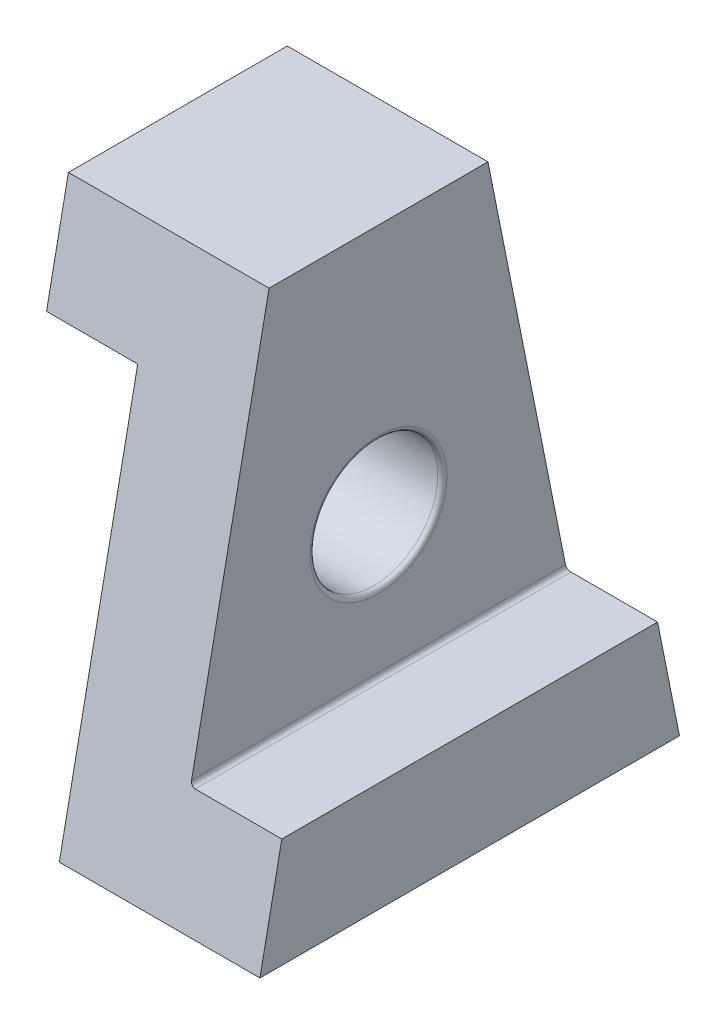
ISO-10303-21;
HEADER;
FILE_DESCRIPTION(('STEP AP214'),'2;1');
FILE_NAME('part.step','',(''),(''),'','','');
FILE_SCHEMA(('AUTOMOTIVE_DESIGN { 1 0 10303 214 1 1 1 1 }'));
ENDSEC;
DATA;
#1=APPLICATION_CONTEXT('core data for automotive mechanical design processes');
#2=APPLICATION_PROTOCOL_DEFINITION('international standard','automotive_design',2000,#1);
#3=PRODUCT_CONTEXT('',#1,'mechanical');
#4=PRODUCT('Part','Part','',(#3));
#5=PRODUCT_RELATED_PRODUCT_CATEGORY('part','',(#4));
#6=PRODUCT_DEFINITION_FORMATION('','',#4);
#7=PRODUCT_DEFINITION_CONTEXT('part definition',#1,'design');
#8=PRODUCT_DEFINITION('design','',#6,#7);
#9=PRODUCT_DEFINITION_SHAPE('','',#8);
#10=(LENGTH_UNIT() NAMED_UNIT(*) SI_UNIT(.MILLI.,.METRE.));
#11=(NAMED_UNIT(*) PLANE_ANGLE_UNIT() SI_UNIT($,.RADIAN.));
#12=(NAMED_UNIT(*) SI_UNIT($,.STERADIAN.) SOLID_ANGLE_UNIT());
#13=UNCERTAINTY_MEASURE_WITH_UNIT(LENGTH_MEASURE(1.E-05),#10,'distance_accuracy_value','');
#14=(GEOMETRIC_REPRESENTATION_CONTEXT(3) GLOBAL_UNCERTAINTY_ASSIGNED_CONTEXT((#13)) GLOBAL_UNIT_ASSIGNED_CONTEXT((#10,
#11,#12)) REPRESENTATION_CONTEXT('',''));
#15=CARTESIAN_POINT('',(0.,0.,0.));
#16=DIRECTION('',(0.,0.,1.));
#17=DIRECTION('',(1.,0.,0.));
#18=AXIS2_PLACEMENT_3D('',#15,#16,#17);
#19=CARTESIAN_POINT('',(0.,43.,46.));
#20=DIRECTION('',(1.,0.,0.));
#21=DIRECTION('',(0.,1.,0.));
#22=AXIS2_PLACEMENT_3D('',#19,#20,#21);
#23=PLANE('',#22);
#24=CARTESIAN_POINT('',(0.,27.5,23.));
#25=DIRECTION('',(1.,0.,0.));
#26=DIRECTION('',(0.,1.,0.));
#27=AXIS2_PLACEMENT_3D('',#24,#25,#26);
#28=CIRCLE('',#27,7.5);
#29=CARTESIAN_POINT('',(0.,35.,23.));
#30=VERTEX_POINT('',#29);
#31=EDGE_CURVE('E147',#30,#30,#28,.T.);
#32=ORIENTED_EDGE('',*,*,#31,.T.);
#33=EDGE_LOOP('',(#32));
#34=FACE_BOUND('',#33,.T.);
#35=DIRECTION('',(0.,0.,-1.));
#36=VECTOR('',#35,1.);
#37=CARTESIAN_POINT('',(0.,0.,46.));
#38=LINE('',#37,#36);
#39=CARTESIAN_POINT('',(0.,0.,46.));
#40=VERTEX_POINT('',#39);
#41=CARTESIAN_POINT('',(0.,0.,0.));
#42=VERTEX_POINT('',#41);
#43=EDGE_CURVE('E134',#40,#42,#38,.T.);
#44=ORIENTED_EDGE('',*,*,#43,.F.);
#45=DIRECTION('',(0.,0.98058067569092,-0.196116135138184));
#46=VECTOR('',#45,1.);
#47=CARTESIAN_POINT('',(0.,41.3461538461538,37.7307692307692));
#48=LINE('',#47,#46);
#49=CARTESIAN_POINT('',(0.,43.,37.4));
#50=VERTEX_POINT('',#49);
#51=EDGE_CURVE('E111',#40,#50,#48,.T.);
#52=ORIENTED_EDGE('',*,*,#51,.T.);
#53=DIRECTION('',(0.,0.,-1.));
#54=VECTOR('',#53,1.);
#55=CARTESIAN_POINT('',(0.,43.,46.));
#56=LINE('',#55,#54);
#57=CARTESIAN_POINT('',(0.,43.,8.6));
#58=VERTEX_POINT('',#57);
#59=EDGE_CURVE('E119',#50,#58,#56,.T.);
#60=ORIENTED_EDGE('',*,*,#59,.T.);
#61=DIRECTION('',(0.,-0.98058067569092,-0.196116135138184));
#62=VECTOR('',#61,1.);
#63=CARTESIAN_POINT('',(0.,50.1923076923077,10.0384615384615));
#64=LINE('',#63,#62);
#65=EDGE_CURVE('E168',#58,#42,#64,.T.);
#66=ORIENTED_EDGE('',*,*,#65,.T.);
#67=EDGE_LOOP('',(#44,#52,#60,#66));
#68=FACE_BOUND('',#67,.T.);
#69=ADVANCED_FACE('F39',(#34,#68),#23,.F.);
#70=CARTESIAN_POINT('',(0.,0.,46.));
#71=DIRECTION('',(0.,1.,0.));
#72=DIRECTION('',(0.,0.,1.));
#73=AXIS2_PLACEMENT_3D('',#70,#71,#72);
#74=PLANE('',#73);
#75=DIRECTION('',(1.,0.,0.));
#76=VECTOR('',#75,1.);
#77=CARTESIAN_POINT('',(0.,0.,0.));
#78=LINE('',#77,#76);
#79=CARTESIAN_POINT('',(22.,0.,0.));
#80=VERTEX_POINT('',#79);
#81=EDGE_CURVE('E117',#42,#80,#78,.T.);
#82=ORIENTED_EDGE('',*,*,#81,.T.);
#83=DIRECTION('',(0.,0.,-1.));
#84=VECTOR('',#83,1.);
#85=CARTESIAN_POINT('',(22.,0.,46.));
#86=LINE('',#85,#84);
#87=CARTESIAN_POINT('',(22.,0.,46.));
#88=VERTEX_POINT('',#87);
#89=EDGE_CURVE('E127',#88,#80,#86,.T.);
#90=ORIENTED_EDGE('',*,*,#89,.F.);
#91=DIRECTION('',(1.,0.,0.));
#92=VECTOR('',#91,1.);
#93=CARTESIAN_POINT('',(0.,0.,46.));
#94=LINE('',#93,#92);
#95=EDGE_CURVE('E107',#40,#88,#94,.T.);
#96=ORIENTED_EDGE('',*,*,#95,.F.);
#97=ORIENTED_EDGE('',*,*,#43,.T.);
#98=EDGE_LOOP('',(#82,#90,#96,#97));
#99=FACE_BOUND('',#98,.T.);
#100=ADVANCED_FACE('F131',(#99),#74,.F.);
#101=CARTESIAN_POINT('',(22.,0.,46.));
#102=DIRECTION('',(-1.,0.,0.));
#103=DIRECTION('',(0.,-1.,0.));
#104=AXIS2_PLACEMENT_3D('',#101,#102,#103);
#105=PLANE('',#104);
#106=DIRECTION('',(0.,0.,-1.));
#107=VECTOR('',#106,1.);
#108=CARTESIAN_POINT('',(22.,12.,46.));
#109=LINE('',#108,#107);
#110=CARTESIAN_POINT('',(22.,12.,43.6));
#111=VERTEX_POINT('',#110);
#112=CARTESIAN_POINT('',(22.,12.,2.4));
#113=VERTEX_POINT('',#112);
#114=EDGE_CURVE('E126',#111,#113,#109,.T.);
#115=ORIENTED_EDGE('',*,*,#114,.F.);
#116=DIRECTION('',(0.,0.98058067569092,-0.196116135138184));
#117=VECTOR('',#116,1.);
#118=CARTESIAN_POINT('',(22.,0.,46.));
#119=LINE('',#118,#117);
#120=EDGE_CURVE('E112',#88,#111,#119,.T.);
#121=ORIENTED_EDGE('',*,*,#120,.F.);
#122=ORIENTED_EDGE('',*,*,#89,.T.);
#123=DIRECTION('',(0.,-0.98058067569092,-0.196116135138184));
#124=VECTOR('',#123,1.);
#125=CARTESIAN_POINT('',(22.,55.,11.));
#126=LINE('',#125,#124);
#127=EDGE_CURVE('E202',#113,#80,#126,.T.);
#128=ORIENTED_EDGE('',*,*,#127,.F.);
#129=EDGE_LOOP('',(#115,#121,#122,#128));
#130=FACE_BOUND('',#129,.T.);
#131=ADVANCED_FACE('F124',(#130),#105,.F.);
#132=CARTESIAN_POINT('',(22.,12.,46.));
#133=DIRECTION('',(0.,-1.,0.));
#134=DIRECTION('',(1.,0.,0.));
#135=AXIS2_PLACEMENT_3D('',#132,#133,#134);
#136=PLANE('',#135);
#137=DIRECTION('',(-1.,0.,0.));
#138=VECTOR('',#137,1.);
#139=CARTESIAN_POINT('',(22.,12.,2.4));
#140=LINE('',#139,#138);
#141=CARTESIAN_POINT('',(12.5,12.,2.4));
#142=VERTEX_POINT('',#141);
#143=EDGE_CURVE('E166',#113,#142,#140,.T.);
#144=ORIENTED_EDGE('',*,*,#143,.T.);
#145=DIRECTION('',(0.,0.,-1.));
#146=VECTOR('',#145,1.);
#147=CARTESIAN_POINT('',(12.5,12.,43.6));
#148=LINE('',#147,#146);
#149=CARTESIAN_POINT('',(12.5,12.,43.6));
#150=VERTEX_POINT('',#149);
#151=EDGE_CURVE('E58',#142,#150,#148,.F.);
#152=ORIENTED_EDGE('',*,*,#151,.T.);
#153=DIRECTION('',(1.,0.,0.));
#154=VECTOR('',#153,1.);
#155=CARTESIAN_POINT('',(22.,12.,43.6));
#156=LINE('',#155,#154);
#157=EDGE_CURVE('E188',#150,#111,#156,.T.);
#158=ORIENTED_EDGE('',*,*,#157,.T.);
#159=ORIENTED_EDGE('',*,*,#114,.T.);
#160=EDGE_LOOP('',(#144,#152,#158,#159));
#161=FACE_BOUND('',#160,.T.);
#162=ADVANCED_FACE('F214',(#161),#136,.F.);
#163=CARTESIAN_POINT('',(12.,12.,46.));
#164=DIRECTION('',(-1.,0.,0.));
#165=DIRECTION('',(0.,0.,1.));
#166=AXIS2_PLACEMENT_3D('',#163,#164,#165);
#167=PLANE('',#166);
#168=CARTESIAN_POINT('',(12.,27.5,23.));
#169=DIRECTION('',(-1.,0.,0.));
#170=DIRECTION('',(0.,0.,1.));
#171=AXIS2_PLACEMENT_3D('',#168,#169,#170);
#172=CIRCLE('',#171,7.5);
#173=CARTESIAN_POINT('',(12.,27.5,30.5));
#174=VERTEX_POINT('',#173);
#175=EDGE_CURVE('E137',#174,#174,#172,.T.);
#176=ORIENTED_EDGE('',*,*,#175,.T.);
#177=EDGE_LOOP('',(#176));
#178=FACE_BOUND('',#177,.T.);
#179=DIRECTION('',(0.,-0.98058067569092,0.196116135138184));
#180=VECTOR('',#179,1.);
#181=CARTESIAN_POINT('',(12.,11.5384615384615,43.6923076923077));
#182=LINE('',#181,#180);
#183=CARTESIAN_POINT('',(12.,55.,35.));
#184=VERTEX_POINT('',#183);
#185=CARTESIAN_POINT('',(12.,12.5,43.5));
#186=VERTEX_POINT('',#185);
#187=EDGE_CURVE('E162',#184,#186,#182,.T.);
#188=ORIENTED_EDGE('',*,*,#187,.T.);
#189=DIRECTION('',(0.,0.,-1.));
#190=VECTOR('',#189,1.);
#191=CARTESIAN_POINT('',(12.,12.5,2.4));
#192=LINE('',#191,#190);
#193=CARTESIAN_POINT('',(12.,12.5,2.5));
#194=VERTEX_POINT('',#193);
#195=EDGE_CURVE('E153',#186,#194,#192,.T.);
#196=ORIENTED_EDGE('',*,*,#195,.T.);
#197=DIRECTION('',(0.,0.98058067569092,0.196116135138184));
#198=VECTOR('',#197,1.);
#199=CARTESIAN_POINT('',(12.,20.3846153846154,4.07692307692307));
#200=LINE('',#199,#198);
#201=CARTESIAN_POINT('',(12.,55.,11.));
#202=VERTEX_POINT('',#201);
#203=EDGE_CURVE('E161',#194,#202,#200,.T.);
#204=ORIENTED_EDGE('',*,*,#203,.T.);
#205=DIRECTION('',(0.,0.,-1.));
#206=VECTOR('',#205,1.);
#207=CARTESIAN_POINT('',(12.,55.,46.));
#208=LINE('',#207,#206);
#209=EDGE_CURVE('E138',#184,#202,#208,.T.);
#210=ORIENTED_EDGE('',*,*,#209,.F.);
#211=EDGE_LOOP('',(#188,#196,#204,#210));
#212=FACE_BOUND('',#211,.T.);
#213=ADVANCED_FACE('F157',(#178,#212),#167,.F.);
#214=CARTESIAN_POINT('',(12.,55.,46.));
#215=DIRECTION('',(0.,-1.,0.));
#216=DIRECTION('',(1.,0.,0.));
#217=AXIS2_PLACEMENT_3D('',#214,#215,#216);
#218=PLANE('',#217);
#219=DIRECTION('',(0.,0.,-1.));
#220=VECTOR('',#219,1.);
#221=CARTESIAN_POINT('',(-10.,55.,46.));
#222=LINE('',#221,#220);
#223=CARTESIAN_POINT('',(-10.,55.,35.));
#224=VERTEX_POINT('',#223);
#225=CARTESIAN_POINT('',(-10.,55.,11.));
#226=VERTEX_POINT('',#225);
#227=EDGE_CURVE('E194',#224,#226,#222,.T.);
#228=ORIENTED_EDGE('',*,*,#227,.F.);
#229=DIRECTION('',(1.,0.,0.));
#230=VECTOR('',#229,1.);
#231=CARTESIAN_POINT('',(-24.,55.,35.));
#232=LINE('',#231,#230);
#233=EDGE_CURVE('E129',#224,#184,#232,.T.);
#234=ORIENTED_EDGE('',*,*,#233,.T.);
#235=ORIENTED_EDGE('',*,*,#209,.T.);
#236=DIRECTION('',(1.,0.,0.));
#237=VECTOR('',#236,1.);
#238=CARTESIAN_POINT('',(-24.,55.,11.));
#239=LINE('',#238,#237);
#240=EDGE_CURVE('E128',#226,#202,#239,.T.);
#241=ORIENTED_EDGE('',*,*,#240,.F.);
#242=EDGE_LOOP('',(#228,#234,#235,#241));
#243=FACE_BOUND('',#242,.T.);
#244=ADVANCED_FACE('F200',(#243),#218,.F.);
#245=CARTESIAN_POINT('',(-10.,55.,46.));
#246=DIRECTION('',(1.,0.,0.));
#247=DIRECTION('',(0.,1.,0.));
#248=AXIS2_PLACEMENT_3D('',#245,#246,#247);
#249=PLANE('',#248);
#250=DIRECTION('',(0.,0.,-1.));
#251=VECTOR('',#250,1.);
#252=CARTESIAN_POINT('',(-10.,43.,46.));
#253=LINE('',#252,#251);
#254=CARTESIAN_POINT('',(-10.,43.,37.4));
#255=VERTEX_POINT('',#254);
#256=CARTESIAN_POINT('',(-10.,43.,8.6));
#257=VERTEX_POINT('',#256);
#258=EDGE_CURVE('E192',#255,#257,#253,.T.);
#259=ORIENTED_EDGE('',*,*,#258,.F.);
#260=DIRECTION('',(0.,0.98058067569092,-0.196116135138184));
#261=VECTOR('',#260,1.);
#262=CARTESIAN_POINT('',(-10.,52.8846153846154,35.4230769230769));
#263=LINE('',#262,#261);
#264=EDGE_CURVE('E182',#255,#224,#263,.T.);
#265=ORIENTED_EDGE('',*,*,#264,.T.);
#266=ORIENTED_EDGE('',*,*,#227,.T.);
#267=DIRECTION('',(0.,-0.98058067569092,-0.196116135138184));
#268=VECTOR('',#267,1.);
#269=CARTESIAN_POINT('',(-10.,61.7307692307692,12.3461538461539));
#270=LINE('',#269,#268);
#271=EDGE_CURVE('E172',#226,#257,#270,.T.);
#272=ORIENTED_EDGE('',*,*,#271,.T.);
#273=EDGE_LOOP('',(#259,#265,#266,#272));
#274=FACE_BOUND('',#273,.T.);
#275=ADVANCED_FACE('F209',(#274),#249,.F.);
#276=CARTESIAN_POINT('',(-10.,43.,46.));
#277=DIRECTION('',(0.,1.,0.));
#278=DIRECTION('',(0.,0.,1.));
#279=AXIS2_PLACEMENT_3D('',#276,#277,#278);
#280=PLANE('',#279);
#281=ORIENTED_EDGE('',*,*,#59,.F.);
#282=DIRECTION('',(-1.,0.,0.));
#283=VECTOR('',#282,1.);
#284=CARTESIAN_POINT('',(-10.,43.,37.4));
#285=LINE('',#284,#283);
#286=EDGE_CURVE('E175',#50,#255,#285,.T.);
#287=ORIENTED_EDGE('',*,*,#286,.T.);
#288=ORIENTED_EDGE('',*,*,#258,.T.);
#289=DIRECTION('',(1.,0.,0.));
#290=VECTOR('',#289,1.);
#291=CARTESIAN_POINT('',(-10.,43.,8.6));
#292=LINE('',#291,#290);
#293=EDGE_CURVE('E199',#257,#58,#292,.T.);
#294=ORIENTED_EDGE('',*,*,#293,.T.);
#295=EDGE_LOOP('',(#281,#287,#288,#294));
#296=FACE_BOUND('',#295,.T.);
#297=ADVANCED_FACE('F213',(#296),#280,.F.);
#298=CARTESIAN_POINT('',(-24.,55.,11.));
#299=DIRECTION('',(0.,-0.196116135138184,0.98058067569092));
#300=DIRECTION('',(0.,-0.98058067569092,-0.196116135138184));
#301=AXIS2_PLACEMENT_3D('',#298,#299,#300);
#302=PLANE('',#301);
#303=ORIENTED_EDGE('',*,*,#127,.T.);
#304=ORIENTED_EDGE('',*,*,#81,.F.);
#305=ORIENTED_EDGE('',*,*,#65,.F.);
#306=ORIENTED_EDGE('',*,*,#293,.F.);
#307=ORIENTED_EDGE('',*,*,#271,.F.);
#308=ORIENTED_EDGE('',*,*,#240,.T.);
#309=ORIENTED_EDGE('',*,*,#203,.F.);
#310=CARTESIAN_POINT('',(12.5,12.5,2.5));
#311=DIRECTION('',(0.,-0.196116135138184,0.98058067569092));
#312=DIRECTION('',(0.,0.98058067569092,0.196116135138184));
#313=AXIS2_PLACEMENT_3D('',#310,#311,#312);
#314=ELLIPSE('',#313,0.509901951359279,0.5);
#315=EDGE_CURVE('E50',#194,#142,#314,.T.);
#316=ORIENTED_EDGE('',*,*,#315,.T.);
#317=ORIENTED_EDGE('',*,*,#143,.F.);
#318=EDGE_LOOP('',(#303,#304,#305,#306,#307,#308,#309,#316,#317));
#319=FACE_BOUND('',#318,.T.);
#320=ADVANCED_FACE('F167',(#319),#302,.F.);
#321=CARTESIAN_POINT('',(-24.,0.,46.));
#322=DIRECTION('',(0.,-0.196116135138184,-0.98058067569092));
#323=DIRECTION('',(0.,0.98058067569092,-0.196116135138184));
#324=AXIS2_PLACEMENT_3D('',#321,#322,#323);
#325=PLANE('',#324);
#326=ORIENTED_EDGE('',*,*,#187,.F.);
#327=ORIENTED_EDGE('',*,*,#233,.F.);
#328=ORIENTED_EDGE('',*,*,#264,.F.);
#329=ORIENTED_EDGE('',*,*,#286,.F.);
#330=ORIENTED_EDGE('',*,*,#51,.F.);
#331=ORIENTED_EDGE('',*,*,#95,.T.);
#332=ORIENTED_EDGE('',*,*,#120,.T.);
#333=ORIENTED_EDGE('',*,*,#157,.F.);
#334=CARTESIAN_POINT('',(12.5,12.5,43.5));
#335=DIRECTION('',(0.,-0.196116135138184,-0.98058067569092));
#336=DIRECTION('',(0.,-0.98058067569092,0.196116135138184));
#337=AXIS2_PLACEMENT_3D('',#334,#335,#336);
#338=ELLIPSE('',#337,0.509901951359279,0.5);
#339=EDGE_CURVE('E11',#150,#186,#338,.T.);
#340=ORIENTED_EDGE('',*,*,#339,.T.);
#341=EDGE_LOOP('',(#326,#327,#328,#329,#330,#331,#332,#333,#340));
#342=FACE_BOUND('',#341,.T.);
#343=ADVANCED_FACE('F109',(#342),#325,.F.);
#344=CARTESIAN_POINT('',(46.,27.5,23.));
#345=DIRECTION('',(-1.,0.,0.));
#346=DIRECTION('',(0.,-1.,0.));
#347=AXIS2_PLACEMENT_3D('',#344,#345,#346);
#348=CYLINDRICAL_SURFACE('',#347,7.);
#349=CARTESIAN_POINT('',(0.5,27.5,23.));
#350=DIRECTION('',(1.,0.,0.));
#351=DIRECTION('',(0.,1.,0.));
#352=AXIS2_PLACEMENT_3D('',#349,#350,#351);
#353=CIRCLE('',#352,7.);
#354=CARTESIAN_POINT('',(0.500000000000001,34.5,23.));
#355=VERTEX_POINT('',#354);
#356=EDGE_CURVE('E150',#355,#355,#353,.F.);
#357=ORIENTED_EDGE('',*,*,#356,.T.);
#358=EDGE_LOOP('',(#357));
#359=FACE_BOUND('',#358,.T.);
#360=CARTESIAN_POINT('',(11.5,27.5,23.));
#361=DIRECTION('',(-1.,0.,0.));
#362=DIRECTION('',(0.,0.,1.));
#363=AXIS2_PLACEMENT_3D('',#360,#361,#362);
#364=CIRCLE('',#363,7.);
#365=CARTESIAN_POINT('',(11.5,27.5,30.));
#366=VERTEX_POINT('',#365);
#367=EDGE_CURVE('E145',#366,#366,#364,.F.);
#368=ORIENTED_EDGE('',*,*,#367,.T.);
#369=EDGE_LOOP('',(#368));
#370=FACE_BOUND('',#369,.T.);
#371=ADVANCED_FACE('F231',(#359,#370),#348,.F.);
#372=CARTESIAN_POINT('',(11.5,27.5,23.));
#373=DIRECTION('',(-1.,0.,0.));
#374=DIRECTION('',(0.,0.,1.));
#375=AXIS2_PLACEMENT_3D('',#372,#373,#374);
#376=TOROIDAL_SURFACE('',#375,7.5,0.5);
#377=ORIENTED_EDGE('',*,*,#367,.F.);
#378=EDGE_LOOP('',(#377));
#379=FACE_BOUND('',#378,.T.);
#380=ORIENTED_EDGE('',*,*,#175,.F.);
#381=EDGE_LOOP('',(#380));
#382=FACE_BOUND('',#381,.T.);
#383=ADVANCED_FACE('F225',(#379,#382),#376,.T.);
#384=CARTESIAN_POINT('',(0.5,27.5,23.));
#385=DIRECTION('',(1.,0.,0.));
#386=DIRECTION('',(0.,1.,0.));
#387=AXIS2_PLACEMENT_3D('',#384,#385,#386);
#388=TOROIDAL_SURFACE('',#387,7.5,0.5);
#389=ORIENTED_EDGE('',*,*,#31,.F.);
#390=EDGE_LOOP('',(#389));
#391=FACE_BOUND('',#390,.T.);
#392=ORIENTED_EDGE('',*,*,#356,.F.);
#393=EDGE_LOOP('',(#392));
#394=FACE_BOUND('',#393,.T.);
#395=ADVANCED_FACE('F220',(#391,#394),#388,.T.);
#396=CARTESIAN_POINT('',(12.5,12.5,46.));
#397=DIRECTION('',(0.,0.,1.));
#398=DIRECTION('',(1.,0.,0.));
#399=AXIS2_PLACEMENT_3D('',#396,#397,#398);
#400=CYLINDRICAL_SURFACE('',#399,0.5);
#401=ORIENTED_EDGE('',*,*,#339,.F.);
#402=ORIENTED_EDGE('',*,*,#151,.F.);
#403=ORIENTED_EDGE('',*,*,#315,.F.);
#404=ORIENTED_EDGE('',*,*,#195,.F.);
#405=EDGE_LOOP('',(#401,#402,#403,#404));
#406=FACE_BOUND('',#405,.T.);
#407=ADVANCED_FACE('F41',(#406),#400,.F.);
#408=CLOSED_SHELL('',(#69,#100,#131,#162,#213,#244,#275,#297,#320,#343,#371,#383,#395,#407));
#409=MANIFOLD_SOLID_BREP('B2',#408);
#410=ADVANCED_BREP_SHAPE_REPRESENTATION('',(#18,#409),#14);
#411=SHAPE_DEFINITION_REPRESENTATION(#9,#410);
ENDSEC;
END-ISO-10303-21;
